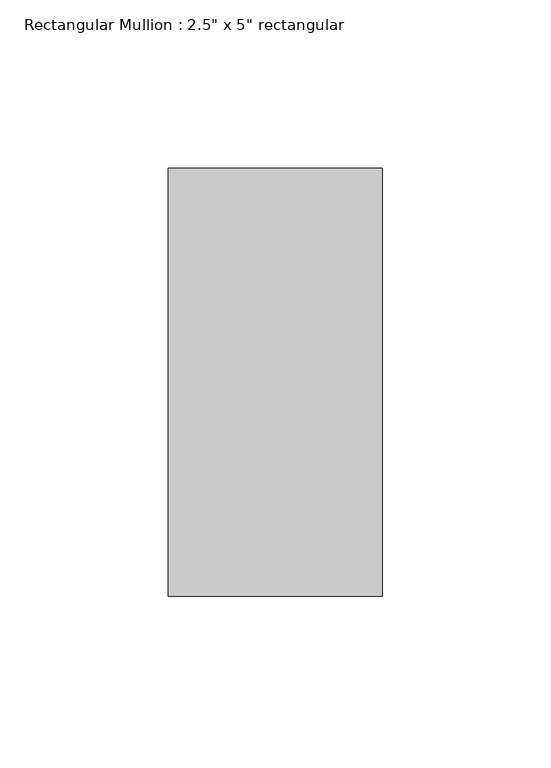
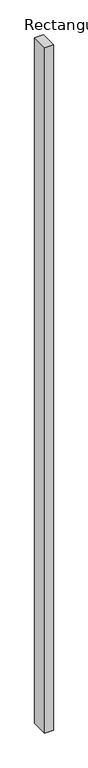
"""IFC4 building model written with IfcOpenShell, lengths in millimetres: member geometry."""

from ifc_helpers import new_model, si_unit, frame, origin, place, context, project, spatial, polyline, outline, extrude, source, transform, mapped, element, save


def member_6c8266e2(model_context):
    return source(origin(), model_context, "Body", "SweptSolid", [
        extrude(outline(polyline([(0.0, 63.5), (0.0, -63.5), (-63.5, -63.5), (-63.5, 63.5), (0.0, 63.5)])), frame((0.0, 0.0, -5317.545847), z_axis=(0.0, 0.0, 1.0), x_axis=(1.0, 0.0, 0.0)), (0.0, 0.0, 1.0), 5317.545847),
    ])


if __name__ == "__main__":
    model = new_model("IFC4")
    model_context = context("Model", 3, world=origin())
    ifc_project = project(units=[si_unit("LENGTHUNIT", "METRE", prefix="MILLI")], contexts=[model_context])
    site = spatial("IfcSite", under=ifc_project)
    building = spatial("IfcBuilding", under=site)
    placement = place(None, origin())
    member_shape = member_6c8266e2(model_context)
    element("IfcMember", 1, ObjectType="Rectangular Mullion : 2.5\" x 5\" rectangular", at=placement, inside=building, context=model_context, shape_type="MappedRepresentation", body=[
        mapped(member_shape, transform((0.0, 0.0, 0.0), x_axis=(1.0, 0.0, 0.0), y_axis=(0.0, 1.0, 0.0), z_axis=(0.0, 0.0, 1.0))),
    ])
    save(model, "model.ifc")

# Revit data of these elements
# Type "Rectangular Mullion : 2.5\" x 5\" rectangular"
#   built-in parameter 1007304 = 0.416667 (stored number, unit not read)
#   built-in parameter 1007301 = 0.104167 (stored number, unit not read)
#   built-in parameter 1007300 = 0.104167 (stored number, unit not read)
# Element 1 (IfcMember, "Rectangular Mullion : 2.5\" x 5\" rectangular")
#   Materials on its faces: "Iron, Ductile"
# Materials
#   "Iron, Ductile": class "Metal", colour RGB 0 0 0, transparency 0, Description = "Ductile cast iron", Cost = 0
